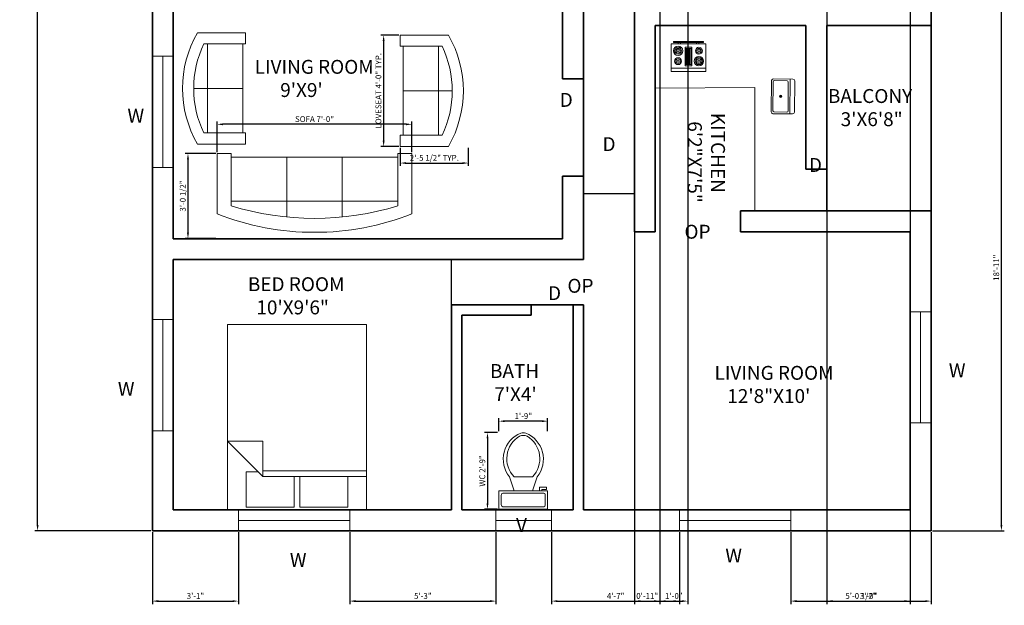
# Model space of a CAD drawing. Units: inches. Extents: x 22580 to 27643822, y 20781 to 31007121.
# Tile 1 of 3: x 27643397 to 27643822, y 31006522 to 31006774. Entities that reach past the tile are written whole.
import ezdxf

# ---------------------------------------------------------------- set-up
doc = ezdxf.new("R2010")
doc.units = ezdxf.units.IN
for name, color, linetype, lineweight in [('A-ANNO-DIMS', 2, 'Continuous', 18), ('A-ANNO-TEXT', 7, 'Continuous', 18), ('A-AREA-IDEN', 7, 'Continuous', 25), ('A-DOOR', 3, 'Continuous', 25), ('A-EQPM', 8, 'Continuous', 18), ('A-FLOR-CASE', 8, 'Continuous', 20), ('A-FLOR-FIXT', 9, 'Continuous', 18), ('A-FURN', 8, 'Continuous', 18), ('A-GLAZ', 4, 'Continuous', 18), ('A-WALL', 7, 'Continuous', 35)]:
    doc.layers.add(name, color=color, linetype=linetype, lineweight=lineweight)
doc.styles.get("Standard").update_dxf_attribs({"font": 'arial.ttf'})
doc.dimstyles.new('ISO-25', dxfattribs={"dimtxt": 2.5, "dimasz": 2.5, "dimexe": 1.25, "dimexo": 0.625, "dimtad": 1, "dimdec": 1, "dimlunit": 3, "dimtxsty": 'Standard', "dimcen": 2.5, "dimadec": 0, "dimazin": 0, "dimtfac": 1, "dimtdec": 1, "dimtmove": 0, "dimatfit": 3, "dimfxl": 1, "dimarcsym": 0})

# ---------------------------------------------------------------- blocks, each defined once
blk = doc.blocks.new('Bed - Queen')
for p, q in [((0, -80.00003), (0, 0)), ((0, 0), (59.99999, 0)), ((59.99999, 0), (59.99999, -80.00003)), ((7.99999, -1.2), (28.79998, -1.2)), ((7.99999, -14.4), (7.99999, -1.2)), ((28.79998, -1.2), (28.79998, -14.4)), ((31.19999, -1.2), (51.99999, -1.2)), ((31.19999, -14.4), (31.19999, -1.2)), ((51.99999, -1.2), (51.99999, -16.4)), ((0, -14.4), (44.8, -14.4)), ((44.8, -16.8), (0, -16.8)), ((59.99999, -29.6), (44.8, -14.4)), ((44.8, -14.4), (44.8, -29.6)), ((51.99999, -16.4), (46.79936, -16.4)), ((44.8, -29.6), (59.99999, -29.6)), ((59.99999, -80.00003), (0, -80.00003))]:
    blk.add_line(p, q)
blk = doc.blocks.new('Toilet - top')
for p, q in [((9.5, -6), (9.5, -2)), ((-8, -8.5), (-8, -8)), ((-7, -8), (-7, -9.5)), ((-4, -8), (-6, -14)), ((4, -8), (6, -14)), ((-10, -8.5), (-8, -8.5)), ((-10, -9.5), (-10, -8.5)), ((-7, -9.5), (-10, -9.5)), ((4, -14), (-4, -14))]:
    blk.add_line(p, q)
blk.add_lwpolyline([(10.5, -8), (10.5, 0), (-10.5, 0), (-10.5, -8)], close=True)
for points in [[(-9.5, -2), (-9.5, -6)], [(8.5, -1), (-8.5, -1)], [(-8.5, -7), (8.5, -7)]]:
    blk.add_lwpolyline(points)
for centre, radius, start, end in [((-8.62, -1.88), 0.884, 81.8699, 188.1301), ((8.62, -1.88), 0.884, 351.8699, 98.1301), ((-8.62, -6.12), 0.884, 171.8699, 278.1301), ((8.62, -6.12), 0.884, 261.8699, 8.1301), ((3.52, -21.58), 12.17, 141.4691, 247.9714), ((4.2, -21.82), 11.33, 136.3677, 238.9468), ((-3.52, -21.58), 12.17, 292.0284, 38.5307), ((-4.2, -21.82), 11.33, 301.053, 43.6321), ((0, -27.88), 4, 245.7318, 294.2682), ((0, -29), 4, 254.8605, 285.1395)]:
    blk.add_arc(centre, radius, start, end)
blk = doc.blocks.new('Range-Oven - 30 in top')
for p, q in [((0, -3), (30, -3)), ((12, -6), (18, -6)), ((13, -20), (13, -6)), ((14, -6), (14, -20)), ((15, -20), (15, -6)), ((16, -6), (16, -20)), ((17, -20), (17, -6)), ((6, -24), (6, -25)), ((8, -25), (8, -24)), ((18, -20), (12, -20)), ((22, -25), (22, -24)), ((24, -24), (24, -25))]:
    blk.add_line(p, q)
for points in [[(0, -24), (0, 0), (30, 0), (30, -24)], [(12, -21), (12, -5), (18, -5), (18, -21)], [(2, -26), (2, -25), (28, -25), (28, -26)]]:
    blk.add_lwpolyline(points, close=True)
for centre, radius in [((6, -9), 4), ((6, -9), 3), ((6, -9), 2), ((6, -9), 1), ((24, -9), 3), ((24, -9), 2), ((24, -9), 1), ((6, -18), 3), ((6, -18), 2), ((24, -18), 4), ((24, -18), 3), ((24, -18), 2), ((6, -18), 1), ((24, -18), 1)]:
    blk.add_circle(centre, radius)
blk = doc.blocks.new('Sink-single - 30 in top')
blk.add_line((-15, -3.999996), (15, -3.999996))
for points in [[(-13.5, 0), (13.5, 0)], [(-15, -18.499996), (-15, -1.5)], [(-13.5, -17.499996), (-13.5, -6.499996)], [(-12.5, -5.499996), (12.5, -5.499996)], [(13.5, -6.499996), (13.5, -17.499996)], [(15, -1.5), (15, -18.499996)], [(13.5, -19.999996), (-13.5, -19.999996)], [(12.5, -18.499996), (-12.5, -18.499996)]]:
    blk.add_lwpolyline(points)
for radius in [1, 0.5]:
    blk.add_circle((0, -11.999996), radius)
for centre, radius, start, end in [((-13.5, -1.5), 1.5, 90, 180), ((-12.5, -6.499996), 1, 90, 180), ((12.5, -6.499996), 1, 0, 90), ((13.5, -1.5), 1.5, 0, 90), ((-13.5, -18.499996), 1.5, 180, 270), ((-12.5, -17.499996), 1, 180, 270), ((12.5, -17.499996), 1, 270, 0), ((13.5, -18.499996), 1.5, 270, 0)]:
    blk.add_arc(centre, radius, start, end)
blk = doc.blocks.new('Sofa - Roundback 7 ft.')
for p, q in [((-12.00002, -32.4421), (-12.00003, -6.5971)), ((11.99997, -32.4421), (11.99998, -6.5971)), ((-36.000027, -34), (-36.000027, -11.4696)), ((35.99998, -34), (35.99998, -11.4696)), ((-35.999844, -13.3819), (35.9998, -13.3819)), ((-36.000027, -32.4421), (35.99998, -32.4421))]:
    blk.add_line(p, q)
for points in [[(-36.000027, -34), (-42.000027, -34), (-42.000027, -8)], [(41.99998, -8), (41.99998, -34), (35.99998, -34)]]:
    blk.add_lwpolyline(points)
for centre, radius, start, end in [((0, -114.25), 114.25, 68.43141, 111.5686), ((-0.00001, -127.1968), 121.1968, 72.72033, 107.2797)]:
    blk.add_arc(centre, radius, start, end)
blk = doc.blocks.new('Sofa - Roundback Loveseat 5 ft.')
for p, q in [((0, -32.44198), (0, -5.99998)), ((-24, -33.99998), (-24, -11.46958)), ((-23.9998, -13.38178), (23.99986, -13.38178)), ((24.00004, -33.99998), (24.00004, -11.46958)), ((-24, -32.44198), (24.00004, -32.44198))]:
    blk.add_line(p, q)
for points in [[(-24, -33.99998), (-30, -33.99998), (-30, -7.99998)], [(30.00004, -7.99998), (30.00004, -33.99998), (24.00004, -33.99998)]]:
    blk.add_lwpolyline(points)
for centre, radius, start, end in [((0, -60.24998), 60.24998, 60.13715, 119.8628), ((0, -61.38438), 55.38444, 64.32083, 115.6792)]:
    blk.add_arc(centre, radius, start, end)
blk = doc.blocks.new('*D10')
at = {"layer": 'A-ANNO-DIMS', "color": 0, "lineweight": -2, "transparency": 16777216}
for p, q in [((27643453.33, 31007083.83), (27643403.16, 31007083.83)), ((27643404.41, 31006556.33), (27643404.41, 31007081.33)), ((27643453.33, 31006553.83), (27643403.16, 31006553.83))]:
    blk.add_line(p, q, dxfattribs=at)
at = {"layer": 'A-ANNO-DIMS', "color": 0, "transparency": 16777216}
for points in [[(27643404, 31007081.33), (27643404.83, 31007081.33), (27643404.41, 31007083.83)], [(27643404, 31006556.33), (27643404.83, 31006556.33), (27643404.41, 31006553.83)]]:
    blk.add_solid(points, dxfattribs=at)
at = {"layer": 'Defpoints', "color": 0, "transparency": 16777216}
for p in [(27643404.41, 31007083.83), (27643453.96, 31007083.83), (27643453.96, 31006553.83)]:
    blk.add_point(p, dxfattribs=at)
at = {"layer": 'A-ANNO-DIMS', "color": 0, "transparency": 16777216, "insert": (27643400.78, 31006818.83), "char_height": 6, "attachment_point": 5, "rotation": 90}
blk.add_mtext('44\'-2"', dxfattribs=at)
blk = doc.blocks.new('WIN-48IN')
for p, q in [((0, 9), (0, 0)), ((48, 9), (48, 0)), ((0, 4.5), (48, 4.5))]:
    blk.add_line(p, q)
blk = doc.blocks.new('VENT-24IN')
for p, q in [((0, 9), (0, 0)), ((24, 9), (24, 0)), ((0, 4.5), (24, 4.5))]:
    blk.add_line(p, q)
blk = doc.blocks.new('*D19')
at = {"layer": 'A-ANNO-DIMS', "color": 0, "lineweight": -2, "transparency": 16777216}
for p, q in [((27643560.31, 31006767.69), (27643552.48, 31006767.69)), ((27643553.73, 31006765.19), (27643553.73, 31006722.19)), ((27643560.31, 31006719.69), (27643552.48, 31006719.69))]:
    blk.add_line(p, q, dxfattribs=at)
at = {"layer": 'A-ANNO-DIMS', "color": 0, "transparency": 16777216}
for points in [[(27643553.32, 31006765.19), (27643554.15, 31006765.19), (27643553.73, 31006767.69)], [(27643553.32, 31006722.19), (27643554.15, 31006722.19), (27643553.73, 31006719.69)]]:
    blk.add_solid(points, dxfattribs=at)
at = {"layer": 'Defpoints', "color": 0, "transparency": 16777216}
for p in [(27643560.93, 31006767.69), (27643553.73, 31006719.69), (27643560.93, 31006719.69)]:
    blk.add_point(p, dxfattribs=at)
at = {"layer": 'A-ANNO-DIMS', "color": 0, "transparency": 16777216, "insert": (27643551.81, 31006743.69), "char_height": 2.5, "attachment_point": 5, "rotation": 90}
blk.add_mtext('LOVESEAT 4\'-0" TYP.', dxfattribs=at)
blk = doc.blocks.new('*D20')
at = {"layer": 'A-ANNO-DIMS', "color": 0, "lineweight": -2, "transparency": 16777216}
for p, q in [((27643560.93, 31006719.06), (27643560.93, 31006711.24)), ((27643590.27, 31006719.06), (27643590.27, 31006711.24)), ((27643563.43, 31006712.49), (27643587.77, 31006712.49))]:
    blk.add_line(p, q, dxfattribs=at)
at = {"layer": 'A-ANNO-DIMS', "color": 0, "transparency": 16777216}
for points in [[(27643563.43, 31006712.91), (27643563.43, 31006712.07), (27643560.93, 31006712.49)], [(27643587.77, 31006712.91), (27643587.77, 31006712.07), (27643590.27, 31006712.49)]]:
    blk.add_solid(points, dxfattribs=at)
at = {"layer": 'Defpoints', "color": 0, "transparency": 16777216}
for p in [(27643560.93, 31006719.69), (27643590.27, 31006719.69), (27643590.27, 31006712.49)]:
    blk.add_point(p, dxfattribs=at)
at = {"layer": 'A-ANNO-DIMS', "color": 0, "transparency": 16777216, "insert": (27643575.6, 31006714.41), "char_height": 2.5, "attachment_point": 5}
blk.add_mtext('2\'-5 1/2" TYP.', dxfattribs=at)
blk = doc.blocks.new('*D21')
at = {"layer": 'A-ANNO-DIMS', "color": 0, "lineweight": -2, "transparency": 16777216}
for p, q in [((27643481.9, 31006717.23), (27643481.9, 31006730.46)), ((27643565.9, 31006717.23), (27643565.9, 31006730.46)), ((27643563.4, 31006729.21), (27643484.4, 31006729.21))]:
    blk.add_line(p, q, dxfattribs=at)
at = {"layer": 'A-ANNO-DIMS', "color": 0, "transparency": 16777216}
for points in [[(27643484.4, 31006729.62), (27643484.4, 31006728.79), (27643481.9, 31006729.21)], [(27643563.4, 31006729.62), (27643563.4, 31006728.79), (27643565.9, 31006729.21)]]:
    blk.add_solid(points, dxfattribs=at)
at = {"layer": 'Defpoints', "color": 0, "transparency": 16777216}
for p in [(27643481.9, 31006729.21), (27643481.9, 31006716.61), (27643565.9, 31006716.61)]:
    blk.add_point(p, dxfattribs=at)
at = {"layer": 'A-ANNO-DIMS', "color": 0, "transparency": 16777216, "insert": (27643523.9, 31006731.13), "char_height": 2.5, "attachment_point": 5}
blk.add_mtext('SOFA 7\'-0"', dxfattribs=at)
blk = doc.blocks.new('*D22')
at = {"layer": 'A-ANNO-DIMS', "color": 0, "lineweight": -2, "transparency": 16777216}
for p, q in [((27643481.27, 31006716.61), (27643468.05, 31006716.61)), ((27643469.3, 31006714.11), (27643469.3, 31006682.44)), ((27643481.27, 31006679.94), (27643468.05, 31006679.94))]:
    blk.add_line(p, q, dxfattribs=at)
at = {"layer": 'A-ANNO-DIMS', "color": 0, "transparency": 16777216}
for points in [[(27643468.88, 31006714.11), (27643469.71, 31006714.11), (27643469.3, 31006716.61)], [(27643468.88, 31006682.44), (27643469.71, 31006682.44), (27643469.3, 31006679.94)]]:
    blk.add_solid(points, dxfattribs=at)
at = {"layer": 'Defpoints', "color": 0, "transparency": 16777216}
for p in [(27643481.9, 31006716.61), (27643469.3, 31006679.94), (27643481.9, 31006679.94)]:
    blk.add_point(p, dxfattribs=at)
at = {"layer": 'A-ANNO-DIMS', "color": 0, "transparency": 16777216, "insert": (27643467.38, 31006698.27), "char_height": 2.5, "attachment_point": 5, "rotation": 90}
blk.add_mtext('3\'-0 1/2"', dxfattribs=at)
blk = doc.blocks.new('*D29')
at = {"layer": 'A-ANNO-DIMS', "color": 0, "lineweight": -2, "transparency": 16777216}
for p, q in [((27643602.88, 31006596.17), (27643597.3, 31006596.17)), ((27643598.55, 31006593.67), (27643598.55, 31006565.63)), ((27643602.88, 31006563.13), (27643597.3, 31006563.13))]:
    blk.add_line(p, q, dxfattribs=at)
at = {"layer": 'A-ANNO-DIMS', "color": 0, "transparency": 16777216}
for points in [[(27643598.13, 31006593.67), (27643598.96, 31006593.67), (27643598.55, 31006596.17)], [(27643598.13, 31006565.63), (27643598.96, 31006565.63), (27643598.55, 31006563.13)]]:
    blk.add_solid(points, dxfattribs=at)
at = {"layer": 'Defpoints', "color": 0, "transparency": 16777216}
for p in [(27643603.5, 31006596.17), (27643598.55, 31006563.13), (27643603.5, 31006563.13)]:
    blk.add_point(p, dxfattribs=at)
at = {"layer": 'A-ANNO-DIMS', "color": 0, "transparency": 16777216, "insert": (27643596.63, 31006579.65), "char_height": 2.5, "attachment_point": 5, "rotation": 90}
blk.add_mtext('WC 2\'-9"', dxfattribs=at)
blk = doc.blocks.new('*D30')
at = {"layer": 'A-ANNO-DIMS', "color": 0, "lineweight": -2, "transparency": 16777216}
for p, q in [((27643603.5, 31006596.8), (27643603.5, 31006602.38)), ((27643624.5, 31006596.8), (27643624.5, 31006602.38)), ((27643622, 31006601.13), (27643606, 31006601.13))]:
    blk.add_line(p, q, dxfattribs=at)
at = {"layer": 'A-ANNO-DIMS', "color": 0, "transparency": 16777216}
for points in [[(27643606, 31006601.55), (27643606, 31006600.71), (27643603.5, 31006601.13)], [(27643622, 31006601.55), (27643622, 31006600.71), (27643624.5, 31006601.13)]]:
    blk.add_solid(points, dxfattribs=at)
at = {"layer": 'Defpoints', "color": 0, "transparency": 16777216}
for p in [(27643603.5, 31006601.13), (27643603.5, 31006596.17), (27643624.5, 31006596.17)]:
    blk.add_point(p, dxfattribs=at)
at = {"layer": 'A-ANNO-DIMS', "color": 0, "transparency": 16777216, "insert": (27643614, 31006603.03), "char_height": 2.5, "attachment_point": 5}
blk.add_mtext('1\'-9"', dxfattribs=at)
blk = doc.blocks.new('*D32')
at = {"layer": 'A-ANNO-DIMS', "color": 0, "lineweight": -2, "transparency": 16777216}
for p, q in [((27643781.58, 31006780.83), (27643821.56, 31006780.83)), ((27643820.31, 31006556.33), (27643820.31, 31006778.33)), ((27643790.58, 31006553.83), (27643821.56, 31006553.83))]:
    blk.add_line(p, q, dxfattribs=at)
at = {"layer": 'A-ANNO-DIMS', "color": 0, "transparency": 16777216}
for points in [[(27643819.89, 31006778.33), (27643820.72, 31006778.33), (27643820.31, 31006780.83)], [(27643819.89, 31006556.33), (27643820.72, 31006556.33), (27643820.31, 31006553.83)]]:
    blk.add_solid(points, dxfattribs=at)
at = {"layer": 'Defpoints', "color": 0, "transparency": 16777216}
for p in [(27643780.96, 31006780.83), (27643820.31, 31006780.83), (27643789.96, 31006553.83)]:
    blk.add_point(p, dxfattribs=at)
at = {"layer": 'A-ANNO-DIMS', "color": 0, "transparency": 16777216, "insert": (27643818.41, 31006667.33), "char_height": 2.5, "attachment_point": 5, "rotation": 90}
blk.add_mtext('18\'-11"', dxfattribs=at)
blk = doc.blocks.new('*D35')
at = {"layer": 'A-ANNO-DIMS', "color": 0, "lineweight": -2, "transparency": 16777216}
for p, q in [((27643639.96, 31006700.01), (27643639.96, 31007115.43)), ((27643642.46, 31007114.18), (27643659.46, 31007114.18)), ((27643661.96, 31006700.01), (27643661.96, 31007115.43))]:
    blk.add_line(p, q, dxfattribs=at)
at = {"layer": 'A-ANNO-DIMS', "color": 0, "transparency": 16777216}
for points in [[(27643642.46, 31007114.6), (27643642.46, 31007113.77), (27643639.96, 31007114.18)], [(27643659.46, 31007114.6), (27643659.46, 31007113.77), (27643661.96, 31007114.18)]]:
    blk.add_solid(points, dxfattribs=at)
at = {"layer": 'Defpoints', "color": 0, "transparency": 16777216}
for p in [(27643661.96, 31007114.18), (27643639.96, 31006699.38), (27643661.96, 31006699.38)]:
    blk.add_point(p, dxfattribs=at)
at = {"layer": 'A-ANNO-DIMS', "color": 0, "transparency": 16777216, "insert": (27643650.96, 31007116.09), "char_height": 2.5, "attachment_point": 5}
blk.add_mtext('1\'-10"', dxfattribs=at)
blk = doc.blocks.new('*D36')
at = {"layer": 'A-ANNO-DIMS', "color": 0, "lineweight": -2, "transparency": 16777216}
for p, q in [((27643744.96, 31006780.21), (27643744.96, 31006522.23)), ((27643780.96, 31006780.21), (27643780.96, 31006522.23)), ((27643747.46, 31006523.48), (27643778.46, 31006523.48))]:
    blk.add_line(p, q, dxfattribs=at)
at = {"layer": 'A-ANNO-DIMS', "color": 0, "transparency": 16777216}
for points in [[(27643747.46, 31006523.9), (27643747.46, 31006523.07), (27643744.96, 31006523.48)], [(27643778.46, 31006523.9), (27643778.46, 31006523.07), (27643780.96, 31006523.48)]]:
    blk.add_solid(points, dxfattribs=at)
at = {"layer": 'Defpoints', "color": 0, "transparency": 16777216}
for p in [(27643744.96, 31006780.83), (27643780.96, 31006780.83), (27643780.96, 31006523.48)]:
    blk.add_point(p, dxfattribs=at)
at = {"layer": 'A-ANNO-DIMS', "color": 0, "transparency": 16777216, "insert": (27643762.96, 31006525.39), "char_height": 2.5, "attachment_point": 5}
blk.add_mtext('3\'-0"', dxfattribs=at)
blk = doc.blocks.new('*D37')
at = {"layer": 'A-ANNO-DIMS', "color": 0, "lineweight": -2, "transparency": 16777216}
for p, q in [((27643672.96, 31006780.21), (27643672.96, 31006522.23)), ((27643684.96, 31006780.21), (27643684.96, 31006522.23)), ((27643675.46, 31006523.48), (27643682.46, 31006523.48))]:
    blk.add_line(p, q, dxfattribs=at)
at = {"layer": 'A-ANNO-DIMS', "color": 0, "transparency": 16777216}
for points in [[(27643675.46, 31006523.9), (27643675.46, 31006523.07), (27643672.96, 31006523.48)], [(27643682.46, 31006523.9), (27643682.46, 31006523.07), (27643684.96, 31006523.48)]]:
    blk.add_solid(points, dxfattribs=at)
at = {"layer": 'Defpoints', "color": 0, "transparency": 16777216}
for p in [(27643672.96, 31006780.83), (27643684.96, 31006780.83), (27643684.96, 31006523.48)]:
    blk.add_point(p, dxfattribs=at)
at = {"layer": 'A-ANNO-DIMS', "color": 0, "transparency": 16777216, "insert": (27643678.96, 31006525.39), "char_height": 2.5, "attachment_point": 5}
blk.add_mtext('1\'-0"', dxfattribs=at)
blk = doc.blocks.new('*D38')
at = {"layer": 'A-ANNO-DIMS', "color": 0, "lineweight": -2, "transparency": 16777216}
for p, q in [((27643661.96, 31006780.21), (27643661.96, 31006522.23)), ((27643672.96, 31006780.21), (27643672.96, 31006522.23)), ((27643664.46, 31006523.48), (27643670.46, 31006523.48))]:
    blk.add_line(p, q, dxfattribs=at)
at = {"layer": 'A-ANNO-DIMS', "color": 0, "transparency": 16777216}
for points in [[(27643664.46, 31006523.9), (27643664.46, 31006523.07), (27643661.96, 31006523.48)], [(27643670.46, 31006523.9), (27643670.46, 31006523.07), (27643672.96, 31006523.48)]]:
    blk.add_solid(points, dxfattribs=at)
at = {"layer": 'Defpoints', "color": 0, "transparency": 16777216}
for p in [(27643661.96, 31006780.83), (27643672.96, 31006780.83), (27643672.96, 31006523.48)]:
    blk.add_point(p, dxfattribs=at)
at = {"layer": 'A-ANNO-DIMS', "color": 0, "transparency": 16777216, "insert": (27643667.46, 31006525.39), "char_height": 2.5, "attachment_point": 5}
blk.add_mtext('0\'-11"', dxfattribs=at)
blk = doc.blocks.new('*D45')
at = {"layer": 'A-ANNO-DIMS', "color": 0, "lineweight": -2, "transparency": 16777216}
for p, q in [((27643453.96, 31006553.21), (27643453.96, 31006522.23)), ((27643491.1, 31006553.21), (27643491.1, 31006522.23)), ((27643456.46, 31006523.48), (27643488.6, 31006523.48))]:
    blk.add_line(p, q, dxfattribs=at)
at = {"layer": 'A-ANNO-DIMS', "color": 0, "transparency": 16777216}
for points in [[(27643456.46, 31006523.9), (27643456.46, 31006523.07), (27643453.96, 31006523.48)], [(27643488.6, 31006523.9), (27643488.6, 31006523.07), (27643491.1, 31006523.48)]]:
    blk.add_solid(points, dxfattribs=at)
at = {"layer": 'Defpoints', "color": 0, "transparency": 16777216}
for p in [(27643453.96, 31006553.83), (27643491.1, 31006553.83), (27643491.1, 31006523.48)]:
    blk.add_point(p, dxfattribs=at)
at = {"layer": 'A-ANNO-DIMS', "color": 0, "transparency": 16777216, "insert": (27643472.53, 31006525.39), "char_height": 2.5, "attachment_point": 5}
blk.add_mtext('3\'-1"', dxfattribs=at)
blk = doc.blocks.new('*D46')
at = {"layer": 'A-ANNO-DIMS', "color": 0, "lineweight": -2, "transparency": 16777216}
for p, q in [((27643539.1, 31006553.21), (27643539.1, 31006522.23)), ((27643602.2, 31006553.21), (27643602.2, 31006522.23)), ((27643541.6, 31006523.48), (27643599.7, 31006523.48))]:
    blk.add_line(p, q, dxfattribs=at)
at = {"layer": 'A-ANNO-DIMS', "color": 0, "transparency": 16777216}
for points in [[(27643541.6, 31006523.9), (27643541.6, 31006523.07), (27643539.1, 31006523.48)], [(27643599.7, 31006523.9), (27643599.7, 31006523.07), (27643602.2, 31006523.48)]]:
    blk.add_solid(points, dxfattribs=at)
at = {"layer": 'Defpoints', "color": 0, "transparency": 16777216}
for p in [(27643539.1, 31006553.83), (27643602.2, 31006553.83), (27643602.2, 31006523.48)]:
    blk.add_point(p, dxfattribs=at)
at = {"layer": 'A-ANNO-DIMS', "color": 0, "transparency": 16777216, "insert": (27643570.65, 31006525.39), "char_height": 2.5, "attachment_point": 5}
blk.add_mtext('5\'-3"', dxfattribs=at)
blk = doc.blocks.new('*D47')
at = {"layer": 'A-ANNO-DIMS', "color": 0, "lineweight": -2, "transparency": 16777216}
for p, q in [((27643626.2, 31006553.21), (27643626.2, 31006522.23)), ((27643681.42, 31006553.21), (27643681.42, 31006522.23)), ((27643628.7, 31006523.48), (27643678.92, 31006523.48))]:
    blk.add_line(p, q, dxfattribs=at)
at = {"layer": 'A-ANNO-DIMS', "color": 0, "transparency": 16777216}
for points in [[(27643628.7, 31006523.9), (27643628.7, 31006523.07), (27643626.2, 31006523.48)], [(27643678.92, 31006523.9), (27643678.92, 31006523.07), (27643681.42, 31006523.48)]]:
    blk.add_solid(points, dxfattribs=at)
at = {"layer": 'Defpoints', "color": 0, "transparency": 16777216}
for p in [(27643626.2, 31006553.83), (27643681.42, 31006553.83), (27643681.42, 31006523.48)]:
    blk.add_point(p, dxfattribs=at)
at = {"layer": 'A-ANNO-DIMS', "color": 0, "transparency": 16777216, "insert": (27643653.81, 31006525.36), "char_height": 2.5, "attachment_point": 5}
blk.add_mtext('4\'-7"', dxfattribs=at)
blk = doc.blocks.new('*D48')
at = {"layer": 'A-ANNO-DIMS', "color": 0, "lineweight": -2, "transparency": 16777216}
for p, q in [((27643729.42, 31006553.21), (27643729.42, 31006522.23)), ((27643789.96, 31006553.21), (27643789.96, 31006522.23)), ((27643731.92, 31006523.48), (27643787.46, 31006523.48))]:
    blk.add_line(p, q, dxfattribs=at)
at = {"layer": 'A-ANNO-DIMS', "color": 0, "transparency": 16777216}
for points in [[(27643731.92, 31006523.9), (27643731.92, 31006523.07), (27643729.42, 31006523.48)], [(27643787.46, 31006523.9), (27643787.46, 31006523.07), (27643789.96, 31006523.48)]]:
    blk.add_solid(points, dxfattribs=at)
at = {"layer": 'Defpoints', "color": 0, "transparency": 16777216}
for p in [(27643729.42, 31006553.83), (27643789.96, 31006553.83), (27643789.96, 31006523.48)]:
    blk.add_point(p, dxfattribs=at)
at = {"layer": 'A-ANNO-DIMS', "color": 0, "transparency": 16777216, "insert": (27643759.69, 31006525.4), "char_height": 2.5, "attachment_point": 5}
blk.add_mtext('5\'-0 1/2"', dxfattribs=at)

msp = doc.modelspace()

# ---------------------------------------------------------------- linework, layer by layer
at = {"layer": 'A-DOOR'}
for p, q in [((27643639.96, 31006699.38), (27643661.96, 31006699.38)), ((27643582.96, 31006651.33), (27643582.96, 31006670.83))]:
    msp.add_line(p, q, dxfattribs=at)
at = {"layer": 'A-FLOR-CASE'}
for p, q in [((27643670.96, 31006744.75), (27643713.92, 31006745.15)), ((27643713.92, 31006745.15), (27643713.92, 31006691.83))]:
    msp.add_line(p, q, dxfattribs=at)
at = {"layer": 'A-WALL'}
for p, q in [((27643453.96, 31006553.83), (27643453.96, 31007083.83)), ((27643789.96, 31007083.83), (27643789.96, 31006553.83)), ((27643639.96, 31006670.83), (27643639.96, 31006960.83)), ((27643630.96, 31006748.84), (27643630.96, 31006951.83)), ((27643661.96, 31006853.83), (27643661.96, 31006682.83)), ((27643462.96, 31006679.83), (27643462.96, 31006787.83)), ((27643670.96, 31006771.83), (27643670.96, 31006682.83)), ((27643735.96, 31006771.83), (27643670.96, 31006771.83)), ((27643735.96, 31006771.83), (27643735.96, 31006709.83)), ((27643744.96, 31006771.83), (27643744.96, 31006691.83)), ((27643789.96, 31006771.83), (27643744.96, 31006771.83)), ((27643630.96, 31006748.84), (27643639.96, 31006748.84)), ((27643744.96, 31006709.83), (27643735.96, 31006709.83)), ((27643630.96, 31006706.84), (27643639.96, 31006706.84)), ((27643630.96, 31006679.83), (27643630.96, 31006706.84)), ((27643713.29, 31006691.83), (27643707.75, 31006691.83)), ((27643707.75, 31006691.83), (27643707.75, 31006682.83)), ((27643735.96, 31006691.83), (27643713.29, 31006691.83)), ((27643789.96, 31006691.83), (27643735.96, 31006691.83)), ((27643462.96, 31006679.83), (27643630.96, 31006679.83)), ((27643670.96, 31006682.83), (27643661.96, 31006682.83)), ((27643707.75, 31006682.83), (27643713.29, 31006682.83)), ((27643713.29, 31006682.83), (27643735.96, 31006682.83)), ((27643780.96, 31006682.83), (27643735.96, 31006682.83)), ((27643780.96, 31006682.83), (27643780.96, 31006562.83)), ((27643462.96, 31006562.83), (27643462.96, 31006670.83)), ((27643462.96, 31006670.83), (27643639.96, 31006670.83)), ((27643582.96, 31006562.83), (27643582.96, 31006651.33)), ((27643639.96, 31006651.33), (27643582.96, 31006651.33)), ((27643617.46, 31006646.83), (27643617.46, 31006651.33)), ((27643635.46, 31006651.33), (27643635.46, 31006562.83)), ((27643639.96, 31006651.33), (27643639.96, 31006562.83)), ((27643587.46, 31006562.83), (27643587.46, 31006646.83)), ((27643617.46, 31006646.83), (27643587.46, 31006646.83)), ((27643582.96, 31006562.83), (27643462.96, 31006562.83)), ((27643635.46, 31006562.83), (27643587.46, 31006562.83)), ((27643780.96, 31006562.83), (27643639.96, 31006562.83)), ((27643780.96, 31006562.83), (27643644.46, 31006562.83)), ((27643789.96, 31006553.83), (27643453.96, 31006553.83))]:
    msp.add_line(p, q, dxfattribs=at)

# ---------------------------------------------------------------- block references
at = {"layer": 'A-EQPM', "xscale": 0.5, "yscale": 0.5, "zscale": 0.5, "rotation": 180}
msp.add_blockref('Range-Oven - 30 in top', (27643692.78, 31006751.96), dxfattribs=at)
at = {"layer": 'A-FLOR-FIXT', "xscale": 0.5, "yscale": 0.5, "zscale": 0.5, "rotation": 269.474623121082}
msp.add_blockref('Sink-single - 30 in top', (27643731.05, 31006741.22), dxfattribs=at)
at = {"layer": 'A-FLOR-FIXT', "rotation": 180}
msp.add_blockref('Toilet - top', (27643614, 31006563.13), dxfattribs=at)
at = {"layer": 'A-FURN', "xscale": 0.8, "yscale": 0.8, "zscale": 0.8}
for p, rotation in [((27643466.96, 31006744.7), 89.99999999999999), ((27643588.13, 31006743.69), 270)]:
    msp.add_blockref('Sofa - Roundback Loveseat 5 ft.', p, dxfattribs=dict(at, rotation=rotation))
at = {"layer": 'A-FURN'}
for name, p, rotation in [('Sofa - Roundback 7 ft.', (27643523.9, 31006682.61), 180), ('Bed - Queen', (27643546.35, 31006562.83), 179.9999999303989)]:
    msp.add_blockref(name, p, dxfattribs=dict(at, rotation=rotation))
at = {"layer": 'A-GLAZ'}
for p, rotation in [((27643462.96, 31006710.61), 90.00000000322179), ((27643462.96, 31006596.98), 90.00000000161089), ((27643780.96, 31006648.35), 270.0000000171828), ((27643729.42, 31006562.83), 180)]:
    msp.add_blockref('WIN-48IN', p, dxfattribs=dict(at, rotation=rotation))
for name, p in [('WIN-48IN', (27643491.1, 31006553.83)), ('VENT-24IN', (27643602.2, 31006553.83))]:
    msp.add_blockref(name, p, dxfattribs=at)

# ---------------------------------------------------------------- texts
at = {"layer": 'A-ANNO-TEXT', "char_height": 6, "attachment_point": 1}
for s, insert in [(' D', (27643629.72, 31006742.75)), ('W', (27643443.19, 31006735.9)), (' D', (27643648.19, 31006723.66)), (' D', (27643737.25, 31006714.67)), ('OP', (27643683.54, 31006685.86)), ('OP', (27643633.04, 31006662.53)), (' D', (27643624.66, 31006659.36)), ('W', (27643797.62, 31006626.02)), ('W', (27643439.04, 31006618.08)), (' V', (27643610.87, 31006559.35)), ('W', (27643513.26, 31006544.24)), ('W', (27643701.17, 31006546.16))]:
    msp.add_mtext_dynamic_manual_height_columns(s, width=6.2882, gutter_width=12.5, heights=[0], dxfattribs=dict(at, insert=insert))
at = {"layer": 'A-AREA-IDEN', "char_height": 6, "attachment_point": 1}
for s, width, heights, insert in [("    LIVING ROOM\\P          9'X9'", 74.9161, [23.22], (27643490.78, 31006757.01)), ('    BALCONY\\P       3\'X6\'8"', 74.9161, [23.22], (27643738.11, 31006744.42)), ('   BED ROOM\\P     10\'X9\'6"', 74.9161, [23.22], (27643489.66, 31006663.22)), ("    BATH \\P     7'X4'", 74.9161, [23.22], (27643592.29, 31006625.76)), ('   LIVING ROOM\\P      12\'8"X10\'', 96.0584, [28.5], (27643691.03, 31006624.97))]:
    msp.add_mtext_dynamic_manual_height_columns(s, width=width, gutter_width=12.5, heights=heights, dxfattribs=dict(at, insert=insert))
at = {"layer": 'A-AREA-IDEN', "insert": (27643701.08, 31006739.65), "char_height": 6, "attachment_point": 1, "rotation": 269.8273}
msp.add_mtext_dynamic_manual_height_columns('   KITCHEN\\P     6\'2"X7\'5"', width=74.9161, gutter_width=12.5, heights=[23.22], dxfattribs=at)

# ---------------------------------------------------------------- dimensions: what is measured, and where the dimension line sits
at = {"layer": 'A-ANNO-DIMS'}
for base, p1, p2, picture, middle in [((27643661.96, 31007114.18), (27643639.96, 31006699.38), (27643661.96, 31006699.38), '*D35', (27643650.96, 31007116.09)), ((27643672.96, 31006523.48), (27643661.96, 31006780.83), (27643672.96, 31006780.83), '*D38', (27643667.46, 31006525.39)), ((27643684.96, 31006523.48), (27643672.96, 31006780.83), (27643684.96, 31006780.83), '*D37', (27643678.96, 31006525.39)), ((27643780.96, 31006523.48), (27643744.96, 31006780.83), (27643780.96, 31006780.83), '*D36', (27643762.96, 31006525.39)), ((27643491.1, 31006523.48), (27643453.96, 31006553.83), (27643491.1, 31006553.83), '*D45', (27643472.53, 31006525.39)), ((27643602.2, 31006523.48), (27643539.1, 31006553.83), (27643602.2, 31006553.83), '*D46', (27643570.65, 31006525.39)), ((27643681.42, 31006523.48), (27643626.2, 31006553.83), (27643681.42, 31006553.83), '*D47', (27643653.81, 31006525.36)), ((27643789.96, 31006523.48), (27643729.42, 31006553.83), (27643789.96, 31006553.83), '*D48', (27643759.69, 31006525.4))]:
    dim = msp.add_linear_dim(base=base, p1=p1, p2=p2, dimstyle='ISO-25', override={"dimdec": 1, "dimlfac": 1, "dimrnd": 0, "dimzin": 1, "dimdsep": 46, "dimlunit": 4, "dimfrac": 2}, dxfattribs=at)
    dim.commit()
    dim.dimension.update_dxf_attribs({"geometry": picture, "text_midpoint": middle})
for base, p1, p2, angle, override, picture, middle in [((27643404.41, 31007083.83), (27643453.96, 31006553.83), (27643453.96, 31007083.83), 90, {"dimtxt": 6, "dimclrd": 0, "dimclre": 0, "dimclrt": 0}, '*D10', (27643400.78, 31006818.83)), ((27643820.31, 31006780.83), (27643789.96, 31006553.83), (27643780.96, 31006780.83), 90, {"dimdec": 1, "dimlfac": 1, "dimrnd": 0, "dimzin": 1, "dimdsep": 46, "dimlunit": 4, "dimfrac": 2}, '*D32', (27643818.41, 31006667.33)), ((27643469.3, 31006679.94), (27643481.9, 31006716.61), (27643481.9, 31006679.94), 270, {"dimdec": 1, "dimlfac": 1, "dimrnd": 0, "dimzin": 1, "dimdsep": 46, "dimlunit": 4, "dimfrac": 2}, '*D22', (27643467.38, 31006698.27)), ((27643603.5, 31006601.13), (27643624.5, 31006596.17), (27643603.5, 31006596.17), 180, {"dimdec": 1, "dimlfac": 1, "dimrnd": 0, "dimzin": 1, "dimdsep": 46, "dimlunit": 4, "dimfrac": 2}, '*D30', (27643614, 31006603.03))]:
    dim = msp.add_linear_dim(base=base, p1=p1, p2=p2, angle=angle, dimstyle='ISO-25', override=override, dxfattribs=at)
    dim.commit()
    dim.dimension.update_dxf_attribs({"geometry": picture, "text_midpoint": middle})
for base, p1, p2, angle, text, picture, middle in [((27643553.73, 31006719.69), (27643560.93, 31006767.69), (27643560.93, 31006719.69), 270, 'LOVESEAT <> TYP.', '*D19', (27643551.81, 31006743.69)), ((27643481.9, 31006729.21), (27643565.9, 31006716.61), (27643481.9, 31006716.61), 180, 'SOFA <>', '*D21', (27643523.9, 31006731.13)), ((27643598.55, 31006563.13), (27643603.5, 31006596.17), (27643603.5, 31006563.13), 270, 'WC <>', '*D29', (27643596.63, 31006579.65))]:
    dim = msp.add_linear_dim(base=base, p1=p1, p2=p2, angle=angle, text=text, dimstyle='ISO-25', override={"dimdec": 1, "dimlfac": 1, "dimrnd": 0, "dimzin": 1, "dimdsep": 46, "dimlunit": 4, "dimfrac": 2}, dxfattribs=at)
    dim.commit()
    dim.dimension.update_dxf_attribs({"geometry": picture, "text_midpoint": middle})
dim = msp.add_linear_dim(base=(27643590.27, 31006712.49), p1=(27643560.93, 31006719.69), p2=(27643590.27, 31006719.69), text='<> TYP.', dimstyle='ISO-25', override={"dimdec": 1, "dimlfac": 1, "dimrnd": 0, "dimzin": 1, "dimdsep": 46, "dimlunit": 4, "dimfrac": 2}, dxfattribs=at)
dim.commit()
dim.dimension.update_dxf_attribs({"geometry": '*D20', "text_midpoint": (27643575.6, 31006714.41)})

doc.saveas('drawing.dxf')
